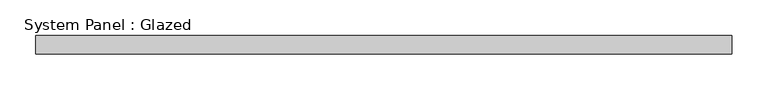
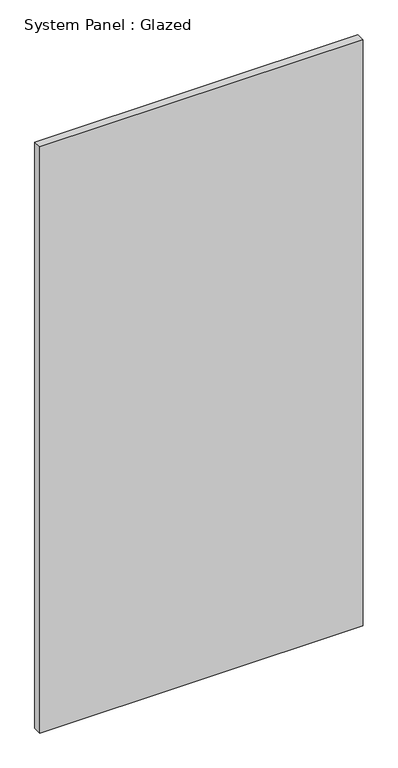
"""IFC4 building model written with IfcOpenShell, lengths in millimetres: plate geometry, System Panel : Glazed."""

from ifc_helpers import new_model, si_unit, origin, origin_with_axes, place, context, project, spatial, polyline, outline, extrude, source, transform, mapped, element, save


def system_panel_glazed_a27b9eb0(model_context):
    return source(origin(), model_context, "Body", "SweptSolid", [
        extrude(outline(polyline([(485.775, 19.05), (-485.775, 19.05), (-485.775, 44.45), (485.775, 44.45), (485.775, 19.05)])), origin_with_axes(), (0.0, 0.0, 1.0), 1861.699716),
    ])


if __name__ == "__main__":
    model = new_model("IFC4")
    model_context = context("Model", 3, world=origin())
    ifc_project = project(units=[si_unit("LENGTHUNIT", "METRE", prefix="MILLI")], contexts=[model_context])
    site = spatial("IfcSite", under=ifc_project)
    building = spatial("IfcBuilding", under=site)
    placement = place(None, origin())
    system_panel_glazed_shape = system_panel_glazed_a27b9eb0(model_context)
    element("IfcPlate", 1, ObjectType="System Panel : Glazed", at=placement, inside=building, context=model_context, shape_type="MappedRepresentation", body=[
        mapped(system_panel_glazed_shape, transform((0.0, 0.0, 0.0), x_axis=(1.0, 0.0, 0.0), y_axis=(0.0, 1.0, 0.0), z_axis=(0.0, 0.0, 1.0))),
    ])
    save(model, "model.ifc")

# Revit data of these elements
# Type "System Panel : Glazed"
#   Construction Type Id = "GSP4R"
#   Analytic Construction = "1/8 in Pilkington single glazing"
#   Visual Light Transmittance = 0.9
#   Solar Heat Gain Coefficient = 0.86
#   Heat Transfer Coefficient (U) = 1.18115 BTU/(h·ft²·°F)
#   Define Thermal Properties by = 1
# Element 1 (IfcPlate, "System Panel : Glazed")
#   Materials on its faces: "Glass"
# Materials
#   "Glass": class "Glass", colour RGB 0 128 192, transparency 0.75, Description = "Soda Lime Glass", Cost = 0
